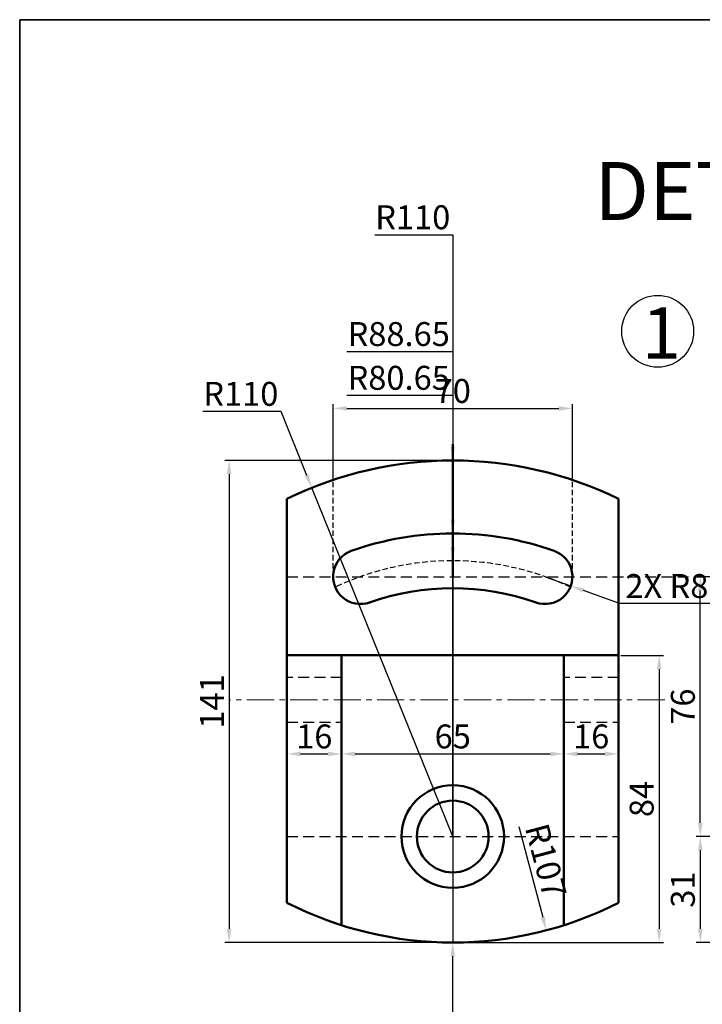
# Model space of a CAD drawing. Units: millimetres. Extents: x -108 to 732, y -172 to 297.
# Tile 2 of 4: x -108 to 91, y 9 to 297. Entities that reach past the tile are written whole.
import ezdxf

# ---------------------------------------------------------------- set-up
doc = ezdxf.new("R2010")
doc.units = ezdxf.units.MM
doc.header["$LTSCALE"] = 0.5
doc.linetypes.add('CENTER', pattern=[50.8, 31.75, -6.35, 6.35, -6.35])
doc.linetypes.add('HIDDEN', pattern=[9.525, 6.35, -3.175])
for name, color, linetype, lineweight in [('M-CNTR', 1, 'CENTER', 18), ('M-DIMS', 2, 'Continuous', 25), ('M-HIDN', 6, 'HIDDEN', 25), ('M-OUTL', 7, 'Continuous', 50), ('M-SYMB', 3, 'Continuous', 25), ('M-TEXT', 3, 'Continuous', 25), ('M-TTLB', 7, 'Continuous', 35)]:
    doc.layers.add(name, color=color, linetype=linetype, lineweight=lineweight)
doc.styles.get("Standard").update_dxf_attribs({"font": 'arial.ttf'})
doc.dimstyles.new('ISO-25', dxfattribs={"dimtxt": 7, "dimasz": 4, "dimexe": 1.25, "dimexo": 0.625, "dimtad": 1, "dimtoh": 1, "dimtxsty": 'Standard', "dimcen": 2.5, "dimadec": 0, "dimazin": 0, "dimtfac": 1, "dimtmove": 0, "dimatfit": 3, "dimfxl": 1, "dimarcsym": 0})

# ---------------------------------------------------------------- blocks, each defined once
blk = doc.blocks.new('*D1')
at = {"layer": 'Defpoints', "color": 0, "ltscale": 0.5, "transparency": 16777216}
for p in [(18.34, 168.21), (-47.07, 27.21), (18.34, 27.21)]:
    blk.add_point(p, dxfattribs=at)
at = {"layer": 'M-DIMS', "color": 0, "lineweight": -2, "ltscale": 0.5, "transparency": 16777216}
for p, q in [((17.72, 168.21), (-48.32, 168.21)), ((-47.07, 164.21), (-47.07, 31.21)), ((17.72, 27.21), (-48.32, 27.21))]:
    blk.add_line(p, q, dxfattribs=at)
at = {"layer": 'M-DIMS', "color": 0, "ltscale": 0.5, "transparency": 16777216}
for points in [[(-47.74, 164.21), (-46.41, 164.21), (-47.07, 168.21)], [(-47.74, 31.21), (-46.41, 31.21), (-47.07, 27.21)]]:
    blk.add_solid(points, dxfattribs=at)
at = {"layer": 'M-DIMS', "color": 0, "ltscale": 0.5, "transparency": 16777216, "insert": (-51.21, 97.71), "char_height": 7, "attachment_point": 5, "rotation": 90}
blk.add_mtext('141', dxfattribs=at)
blk = doc.blocks.new('*D9')
at = {"layer": 'Defpoints', "color": 0, "ltscale": 0.5, "transparency": 16777216}
for p in [(119.6, 58.21), (90.76, 27.21), (119.6, 27.21)]:
    blk.add_point(p, dxfattribs=at)
at = {"layer": 'M-DIMS', "color": 0, "lineweight": -2, "ltscale": 0.5, "transparency": 16777216}
for p, q in [((118.97, 58.21), (89.51, 58.21)), ((90.76, 54.21), (90.76, 31.21)), ((118.97, 27.21), (89.51, 27.21))]:
    blk.add_line(p, q, dxfattribs=at)
at = {"layer": 'M-DIMS', "color": 0, "ltscale": 0.5, "transparency": 16777216}
for points in [[(90.09, 54.21), (91.43, 54.21), (90.76, 58.21)], [(90.09, 31.21), (91.43, 31.21), (90.76, 27.21)]]:
    blk.add_solid(points, dxfattribs=at)
at = {"layer": 'M-DIMS', "color": 0, "ltscale": 0.5, "transparency": 16777216, "insert": (86.56, 42.71), "char_height": 7, "attachment_point": 5, "rotation": 90}
blk.add_mtext('31', dxfattribs=at)
blk = doc.blocks.new('*D10')
at = {"layer": 'Defpoints', "color": 0, "ltscale": 0.5, "transparency": 16777216}
for p in [(90.76, 134.21), (119.6, 134.21), (90.76, 58.21)]:
    blk.add_point(p, dxfattribs=at)
at = {"layer": 'M-DIMS', "color": 0, "lineweight": -2, "ltscale": 0.5, "transparency": 16777216}
for p, q in [((118.97, 134.21), (89.51, 134.21)), ((90.76, 62.21), (90.76, 130.21)), ((90.14, 58.21), (89.51, 58.21))]:
    blk.add_line(p, q, dxfattribs=at)
at = {"layer": 'M-DIMS', "color": 0, "ltscale": 0.5, "transparency": 16777216}
for points in [[(90.09, 130.21), (91.43, 130.21), (90.76, 134.21)], [(90.09, 62.21), (91.43, 62.21), (90.76, 58.21)]]:
    blk.add_solid(points, dxfattribs=at)
at = {"layer": 'M-DIMS', "color": 0, "ltscale": 0.5, "transparency": 16777216, "insert": (86.56, 96.21), "char_height": 7, "attachment_point": 5, "rotation": 90}
blk.add_mtext('76', dxfattribs=at)
blk = doc.blocks.new('*D14')
at = {"layer": 'Defpoints', "color": 0, "ltscale": 0.5, "transparency": 16777216}
for p in [(53.34, 183.42), (-16.66, 162.5), (53.34, 162.5)]:
    blk.add_point(p, dxfattribs=at)
at = {"layer": 'M-DIMS', "color": 0, "lineweight": -2, "ltscale": 0.5, "transparency": 16777216}
for p, q in [((-16.66, 163.12), (-16.66, 184.67)), ((53.34, 163.12), (53.34, 184.67)), ((-12.66, 183.42), (49.34, 183.42))]:
    blk.add_line(p, q, dxfattribs=at)
at = {"layer": 'M-DIMS', "color": 0, "ltscale": 0.5, "transparency": 16777216}
for points in [[(-12.66, 184.08), (-12.66, 182.75), (-16.66, 183.42)], [(49.34, 184.08), (49.34, 182.75), (53.34, 183.42)]]:
    blk.add_solid(points, dxfattribs=at)
at = {"layer": 'M-DIMS', "color": 0, "ltscale": 0.5, "transparency": 16777216, "insert": (18.34, 187.62), "char_height": 7, "attachment_point": 5}
blk.add_mtext('70', dxfattribs=at)
blk = doc.blocks.new('*D15')
at = {"layer": 'Defpoints', "color": 0, "ltscale": 0.5, "transparency": 16777216}
for p in [(-14.16, 84.62), (50.84, 84.62), (50.84, 82.38)]:
    blk.add_point(p, dxfattribs=at)
at = {"layer": 'M-DIMS', "color": 0, "lineweight": -2, "ltscale": 0.5, "transparency": 16777216}
for p, q in [((-14.16, 84), (-14.16, 81.13)), ((50.84, 84), (50.84, 81.13)), ((-10.16, 82.38), (46.84, 82.38))]:
    blk.add_line(p, q, dxfattribs=at)
at = {"layer": 'M-DIMS', "color": 0, "ltscale": 0.5, "transparency": 16777216}
for points in [[(-10.16, 83.05), (-10.16, 81.71), (-14.16, 82.38)], [(46.84, 83.05), (46.84, 81.71), (50.84, 82.38)]]:
    blk.add_solid(points, dxfattribs=at)
at = {"layer": 'M-DIMS', "color": 0, "ltscale": 0.5, "transparency": 16777216, "insert": (18.34, 86.58), "char_height": 7, "attachment_point": 5}
blk.add_mtext('65', dxfattribs=at)
blk = doc.blocks.new('*D16')
at = {"layer": 'Defpoints', "color": 0, "ltscale": 0.5, "transparency": 16777216}
for p in [(-30.16, 82.38), (-14.16, 82.38), (-14.16, 82.38)]:
    blk.add_point(p, dxfattribs=at)
at = {"layer": 'M-DIMS', "color": 0, "lineweight": -2, "ltscale": 0.5, "transparency": 16777216}
for p, q in [((-30.16, 83), (-30.16, 83.63)), ((-14.16, 83), (-14.16, 83.63)), ((-26.16, 82.38), (-18.16, 82.38))]:
    blk.add_line(p, q, dxfattribs=at)
at = {"layer": 'M-DIMS', "color": 0, "ltscale": 0.5, "transparency": 16777216}
for points in [[(-26.16, 83.05), (-26.16, 81.71), (-30.16, 82.38)], [(-18.16, 83.05), (-18.16, 81.71), (-14.16, 82.38)]]:
    blk.add_solid(points, dxfattribs=at)
at = {"layer": 'M-DIMS', "color": 0, "ltscale": 0.5, "transparency": 16777216, "insert": (-22.16, 86.58), "char_height": 7, "attachment_point": 5}
blk.add_mtext('16', dxfattribs=at)
blk = doc.blocks.new('*D17')
at = {"layer": 'Defpoints', "color": 0, "ltscale": 0.5, "transparency": 16777216}
for p in [(50.84, 82.38), (66.84, 82.38), (66.84, 82.38)]:
    blk.add_point(p, dxfattribs=at)
at = {"layer": 'M-DIMS', "color": 0, "lineweight": -2, "ltscale": 0.5, "transparency": 16777216}
for p, q in [((50.84, 83), (50.84, 83.63)), ((66.84, 83), (66.84, 83.63)), ((54.84, 82.38), (62.84, 82.38))]:
    blk.add_line(p, q, dxfattribs=at)
at = {"layer": 'M-DIMS', "color": 0, "ltscale": 0.5, "transparency": 16777216}
for points in [[(54.84, 83.05), (54.84, 81.71), (50.84, 82.38)], [(62.84, 83.05), (62.84, 81.71), (66.84, 82.38)]]:
    blk.add_solid(points, dxfattribs=at)
at = {"layer": 'M-DIMS', "color": 0, "ltscale": 0.5, "transparency": 16777216, "insert": (58.84, 86.58), "char_height": 7, "attachment_point": 5}
blk.add_mtext('16', dxfattribs=at)
blk = doc.blocks.new('*D18')
at = {"layer": 'Defpoints', "color": 0, "ltscale": 0.5, "transparency": 16777216}
for p in [(18.34, 134.21), (45.68, 30.77)]:
    blk.add_point(p, dxfattribs=at)
at = {"layer": 'M-DIMS', "color": 0, "lineweight": -2, "ltscale": 0.5, "transparency": 16777216}
blk.add_line((37.65, 61.15), (44.66, 34.63), dxfattribs=at)
at = {"layer": 'M-DIMS', "color": 0, "ltscale": 0.5, "transparency": 16777216}
blk.add_solid([(45.3, 34.8), (44.01, 34.46), (45.68, 30.77)], dxfattribs=at)
at = {"layer": 'M-DIMS', "color": 0, "ltscale": 0.5, "transparency": 16777216, "insert": (44.7, 50.9), "char_height": 7, "attachment_point": 5, "rotation": 284.804}
blk.add_mtext('R107', dxfattribs=at)
blk = doc.blocks.new('*D19')
at = {"layer": 'Defpoints', "color": 0, "ltscale": 0.5, "transparency": 16777216}
for p in [(-22.89, 160.2), (18.34, 58.21)]:
    blk.add_point(p, dxfattribs=at)
at = {"layer": 'M-DIMS', "color": 0, "lineweight": -2, "ltscale": 0.5, "transparency": 16777216}
for p, q in [((-54.72, 182.58), (-31.93, 182.58)), ((-31.93, 182.58), (-24.39, 163.91)), ((18.34, 58.21), (-22.89, 160.2))]:
    blk.add_line(p, q, dxfattribs=at)
at = {"layer": 'M-DIMS', "color": 0, "ltscale": 0.5, "transparency": 16777216}
blk.add_solid([(-23.77, 164.15), (-25, 163.66), (-22.89, 160.2)], dxfattribs=at)
at = {"layer": 'M-DIMS', "color": 0, "ltscale": 0.5, "transparency": 16777216, "insert": (-43.65, 186.77), "char_height": 7, "attachment_point": 5}
blk.add_mtext('R110', dxfattribs=at)
blk = doc.blocks.new('*D22')
at = {"layer": 'Defpoints', "color": 0, "ltscale": 0.5, "transparency": 16777216}
for p in [(66.84, 111.21), (18.34, 27.21), (78.71, 27.21)]:
    blk.add_point(p, dxfattribs=at)
at = {"layer": 'M-DIMS', "color": 0, "lineweight": -2, "ltscale": 0.5, "transparency": 16777216}
for p, q in [((67.47, 111.21), (79.96, 111.21)), ((78.71, 107.21), (78.71, 31.21)), ((18.97, 27.21), (79.96, 27.21))]:
    blk.add_line(p, q, dxfattribs=at)
at = {"layer": 'M-DIMS', "color": 0, "ltscale": 0.5, "transparency": 16777216}
for points in [[(78.05, 107.21), (79.38, 107.21), (78.71, 111.21)], [(78.05, 31.21), (79.38, 31.21), (78.71, 27.21)]]:
    blk.add_solid(points, dxfattribs=at)
at = {"layer": 'M-DIMS', "color": 0, "ltscale": 0.5, "transparency": 16777216, "insert": (74.51, 69.21), "char_height": 7, "attachment_point": 5, "rotation": 90}
blk.add_mtext('84', dxfattribs=at)
blk = doc.blocks.new('*D52')
at = {"layer": 'Defpoints', "color": 0, "ltscale": 0.5, "transparency": 16777216}
for p in [(18.34, 146.87), (18.34, 58.21)]:
    blk.add_point(p, dxfattribs=at)
at = {"layer": 'M-DIMS', "color": 0, "lineweight": -2, "ltscale": 0.5, "transparency": 16777216}
for p, q in [((-12.66, 200.06), (18.34, 200.06)), ((18.34, 200.06), (18.34, 150.87)), ((18.34, 58.21), (18.34, 146.87))]:
    blk.add_line(p, q, dxfattribs=at)
at = {"layer": 'M-DIMS', "color": 0, "ltscale": 0.5, "transparency": 16777216}
blk.add_solid([(19.01, 150.87), (17.67, 150.87), (18.34, 146.87)], dxfattribs=at)
at = {"layer": 'M-DIMS', "color": 0, "ltscale": 0.5, "transparency": 16777216, "insert": (2.53, 204.26), "char_height": 7, "attachment_point": 5}
blk.add_mtext('R88.65', dxfattribs=at)
blk = doc.blocks.new('*D53')
at = {"layer": 'Defpoints', "color": 0, "ltscale": 0.5, "transparency": 16777216}
for p in [(18.34, 138.87), (18.34, 58.21)]:
    blk.add_point(p, dxfattribs=at)
at = {"layer": 'M-DIMS', "color": 0, "lineweight": -2, "ltscale": 0.5, "transparency": 16777216}
for p, q in [((-12.66, 187.26), (18.34, 187.26)), ((18.34, 187.26), (18.34, 142.87)), ((18.34, 58.21), (18.34, 138.87))]:
    blk.add_line(p, q, dxfattribs=at)
at = {"layer": 'M-DIMS', "color": 0, "ltscale": 0.5, "transparency": 16777216}
blk.add_solid([(19.01, 142.87), (17.67, 142.87), (18.34, 138.87)], dxfattribs=at)
at = {"layer": 'M-DIMS', "color": 0, "ltscale": 0.5, "transparency": 16777216, "insert": (2.53, 191.46), "char_height": 7, "attachment_point": 5}
blk.add_mtext('R80.65', dxfattribs=at)
blk = doc.blocks.new('*D54')
at = {"layer": 'Defpoints', "color": 0, "ltscale": 0.5, "transparency": 16777216}
for p in [(45.34, 134.21), (52.87, 131.51)]:
    blk.add_point(p, dxfattribs=at)
at = {"layer": 'M-DIMS', "color": 0, "lineweight": -2, "ltscale": 0.5, "transparency": 16777216}
for p, q in [((45.34, 134.21), (52.87, 131.51)), ((67.12, 126.38), (56.63, 130.15)), ((94.21, 126.38), (67.12, 126.38))]:
    blk.add_line(p, q, dxfattribs=at)
at = {"layer": 'M-DIMS', "color": 0, "ltscale": 0.5, "transparency": 16777216}
blk.add_solid([(56.86, 130.78), (56.41, 129.53), (52.87, 131.51)], dxfattribs=at)
at = {"layer": 'M-DIMS', "color": 0, "ltscale": 0.5, "transparency": 16777216, "insert": (80.98, 130.58), "char_height": 7, "attachment_point": 5}
blk.add_mtext('2X R8', dxfattribs=at)
blk = doc.blocks.new('*D55')
at = {"layer": 'Defpoints', "color": 0, "ltscale": 0.5, "transparency": 16777216}
for p in [(18.34, 168.21), (18.34, 58.21)]:
    blk.add_point(p, dxfattribs=at)
at = {"layer": 'M-DIMS', "color": 0, "lineweight": -2, "ltscale": 0.5, "transparency": 16777216}
for p, q in [((-4.43, 234.21), (18.34, 234.21)), ((18.34, 234.21), (18.34, 172.21)), ((18.34, 58.21), (18.34, 168.21))]:
    blk.add_line(p, q, dxfattribs=at)
at = {"layer": 'M-DIMS', "color": 0, "ltscale": 0.5, "transparency": 16777216}
blk.add_solid([(19.01, 172.21), (17.67, 172.21), (18.34, 168.21)], dxfattribs=at)
at = {"layer": 'M-DIMS', "color": 0, "ltscale": 0.5, "transparency": 16777216, "insert": (6.64, 238.41), "char_height": 7, "attachment_point": 5}
blk.add_mtext('R110', dxfattribs=at)
blk = doc.blocks.new('*D56')
at = {"layer": 'Defpoints', "color": 0, "ltscale": 0.5, "transparency": 16777216}
for p in [(18.34, 134.21), (18.34, 27.21)]:
    blk.add_point(p, dxfattribs=at)
at = {"layer": 'M-DIMS', "color": 0, "lineweight": -2, "ltscale": 0.5, "transparency": 16777216}
for p, q in [((18.34, 134.21), (18.34, 27.21)), ((18.34, -36.99), (18.34, 23.21)), ((-4.45, -36.99), (18.34, -36.99))]:
    blk.add_line(p, q, dxfattribs=at)
at = {"layer": 'M-DIMS', "color": 0, "ltscale": 0.5, "transparency": 16777216}
blk.add_solid([(17.67, 23.21), (19.01, 23.21), (18.34, 27.21)], dxfattribs=at)
at = {"layer": 'M-DIMS', "color": 0, "ltscale": 0.5, "transparency": 16777216, "insert": (6.63, -32.79), "char_height": 7, "attachment_point": 5}
blk.add_mtext('R107', dxfattribs=at)

msp = doc.modelspace()

# ---------------------------------------------------------------- linework, layer by layer
at = {"layer": 'M-CNTR'}
msp.add_line((18.34, 27.214), (18.34, 168.214), dxfattribs=at)
at = {"layer": 'M-CNTR', "ltscale": 0.5}
msp.add_line((80.364, 98.214), (-46.955, 98.214), dxfattribs=at)
at = {"layer": 'M-HIDN', "ltscale": 0.5}
for p, q in [((-16.66, 134.214), (-16.66, 172.981)), ((53.34, 134.214), (53.34, 172.981))]:
    msp.add_line(p, q, dxfattribs=at)
at = {"layer": 'M-HIDN'}
for p, q in [((-30.16, 134.214), (136.598, 134.214)), ((-14.16, 104.714), (-30.16, 104.714)), ((66.84, 104.714), (50.84, 104.714)), ((-30.16, 91.714), (-14.16, 91.714)), ((50.84, 91.714), (66.84, 91.714)), ((-30.16, 58.214), (66.84, 58.214))]:
    msp.add_line(p, q, dxfattribs=at)
at = {"layer": 'M-HIDN', "ltscale": 0.5}
msp.add_arc((18.34, 58.214), 80.654, 64.75628, 115.24372, dxfattribs=at)
at = {"layer": 'M-OUTL', "ltscale": 0.5}
msp.add_line((18.34, 134.214), (18.34, 172.981), dxfattribs=at)
at = {"layer": 'M-OUTL'}
for p, q in [((-30.16, 38.838), (-30.16, 156.945)), ((66.84, 38.838), (66.84, 156.945)), ((66.84, 111.214), (-30.16, 111.214)), ((-14.16, 32.27), (-14.16, 111.214)), ((50.84, 32.27), (50.84, 111.214))]:
    msp.add_line(p, q, dxfattribs=at)
for radius in [15, 10.5]:
    msp.add_circle((18.34, 58.214), radius, dxfattribs=at)
for centre, radius, start, end in [((18.34, 58.214), 110, 63.8381, 116.1619), ((18.34, 134.214), 107, 243.04626, 296.95374)]:
    msp.add_arc(centre, radius, start, end, dxfattribs=at)
at = {"layer": 'M-OUTL', "ltscale": 0.5}
for centre, radius, start, end in [((18.34, 58.214), 88.654, 70.44175, 109.55825), ((-8.66, 134.214), 8, 109.55825, 289.99001), ((45.34, 134.214), 8, 250.00999, 70.44175), ((18.34, 58.214), 72.654, 70.39421, 109.60579)]:
    msp.add_arc(centre, radius, start, end, dxfattribs=at)
at = {"layer": 'M-SYMB', "ltscale": 0.5}
msp.add_circle((78.297, 205.962), 10.513, dxfattribs=at)
at = {"layer": 'M-TTLB', "ltscale": 0.5}
msp.add_lwpolyline([(-108.335, 297.096), (732.37, 297.096), (732.37, -172.452), (-108.335, -172.452)], close=True, dxfattribs=at)

# ---------------------------------------------------------------- texts
at = {"layer": 'M-TEXT', "ltscale": 0.5, "attachment_point": 1}
for s, width, heights, insert, char_height in [('\\pxqc;DETAILS OF CLAPPER BLOCK', 372.02553, [0], (28.998, 255.491), 17), ('1', 20, [1.225], (73.694, 212.97), 15)]:
    msp.add_mtext_dynamic_manual_height_columns(s, width=width, gutter_width=12.5, heights=heights, dxfattribs=dict(at, insert=insert, char_height=char_height))

# ---------------------------------------------------------------- dimensions: what is measured, and where the dimension line sits
at = {"layer": 'M-DIMS', "ltscale": 0.5}
for center, mpoint, override, picture, middle in [((18.34, 58.214), (18.34, 168.214), {"dimdec": 0, "dimlfac": 1, "dimrnd": 0, "dimzin": 0, "dimdsep": 46, "dimlunit": 2}, '*D55', (6.644, 234.214)), ((18.34, 58.214), (18.34, 146.868), {"dimdec": 2, "dimlfac": 1, "dimrnd": 0, "dimzin": 0, "dimdsep": 46, "dimlunit": 2}, '*D52', (2.528, 200.06)), ((18.34, 58.214), (18.34, 138.868), {"dimdec": 2, "dimlfac": 1, "dimrnd": 0, "dimzin": 0, "dimdsep": 46, "dimlunit": 2}, '*D53', (2.528, 187.261)), ((18.34, 58.214), (-22.886, 160.197), {"dimclrd": 0, "dimclre": 0, "dimclrt": 0}, '*D19', (-43.648, 182.576)), ((18.34, 134.214), (18.34, 27.214), {"dimdec": 0, "dimlfac": 1, "dimrnd": 0, "dimzin": 0, "dimdsep": 46, "dimlunit": 2}, '*D56', (6.632, -36.986)), ((18.34, 134.214), (45.68, 30.766), {"dimclrd": 0, "dimclre": 0, "dimclrt": 0}, '*D18', (40.643, 49.827))]:
    dim = msp.add_radius_dim(center=center, mpoint=mpoint, dimstyle='ISO-25', override=override, dxfattribs=at)
    dim.commit()
    dim.dimension.update_dxf_attribs({"geometry": picture, "text_midpoint": middle, "dimtype": 164})
for base, p1, p2, picture, middle in [((53.34, 183.418), (-16.66, 162.498), (53.34, 162.498), '*D14', (18.34, 187.617)), ((-14.16, 82.379), (-30.16, 82.379), (-14.16, 82.379), '*D16', (-22.16, 86.578)), ((50.84, 82.379), (-14.16, 84.623), (50.84, 84.623), '*D15', (18.34, 86.578)), ((66.84, 82.379), (50.84, 82.379), (66.84, 82.379), '*D17', (58.84, 86.578))]:
    dim = msp.add_linear_dim(base=base, p1=p1, p2=p2, dimstyle='ISO-25', override={"dimclrd": 0, "dimclre": 0, "dimclrt": 0}, dxfattribs=at)
    dim.commit()
    dim.dimension.update_dxf_attribs({"geometry": picture, "text_midpoint": middle})
for base, p1, p2, picture, middle in [((-47.075, 27.214), (18.34, 168.214), (18.34, 27.214), '*D1', (-51.214, 97.714)), ((90.761, 134.214), (90.761, 58.214), (119.598, 134.214), '*D10', (86.562, 96.214)), ((78.713, 27.214), (66.84, 111.214), (18.34, 27.214), '*D22', (74.514, 69.214)), ((90.761, 27.214), (119.598, 58.214), (119.598, 27.214), '*D9', (86.559, 42.714))]:
    dim = msp.add_linear_dim(base=base, p1=p1, p2=p2, angle=90, dimstyle='ISO-25', override={"dimclrd": 0, "dimclre": 0, "dimclrt": 0}, dxfattribs=at)
    dim.commit()
    dim.dimension.update_dxf_attribs({"geometry": picture, "text_midpoint": middle})
dim = msp.add_radius_dim(center=(45.34, 134.214), mpoint=(52.869, 131.508), text='2X <>', dimstyle='ISO-25', override={"dimdec": 0, "dimlfac": 1, "dimrnd": 0, "dimzin": 0, "dimdsep": 46, "dimlunit": 2}, dxfattribs=at)
dim.commit()
dim.dimension.update_dxf_attribs({"geometry": '*D54', "text_midpoint": (80.98, 130.582)})

doc.saveas('drawing.dxf')
